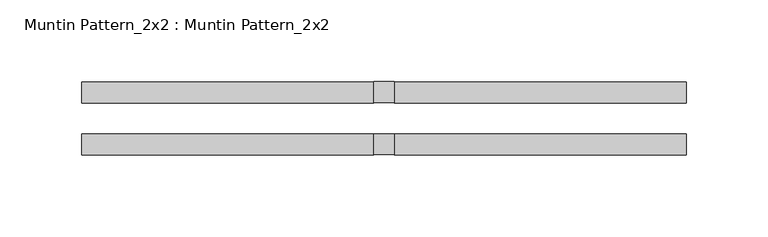
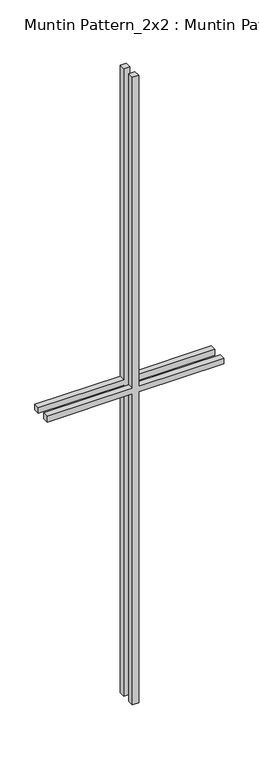
"""IFC4 building model written with IfcOpenShell, lengths in millimetres: proxy geometry, Muntin Pattern_2x2 : Muntin Pattern_2x2."""

from ifc_helpers import new_model, si_unit, frame, origin, place, context, project, spatial, polyline, outline, extrude, source, transform, mapped, element, save


def muntin_pattern_2x2_muntin_pattern_2x2_218eda85(model_context):
    return source(origin(), model_context, "Body", "SweptSolid", [
        extrude(outline(polyline([(698.5, -6.35), (698.5, -184.15), (685.8, -184.15), (685.8, -6.35), (0.0, -6.35), (0.0, 6.35), (685.8, 6.35), (685.8, 184.15), (698.5, 184.15), (698.5, 6.35), (1384.3, 6.35), (1384.3, -6.35), (698.5, -6.35)])), frame((0.0, -22.225, 0.0), z_axis=(0.0, 1.0, 0.0), x_axis=(0.0, 0.0, 1.0)), (0.0, 0.0, 1.0), 12.7),
        extrude(outline(polyline([(698.5, -6.35), (698.5, -184.15), (685.8, -184.15), (685.8, -6.35), (0.0, -6.35), (0.0, 6.35), (685.8, 6.35), (685.8, 184.15), (698.5, 184.15), (698.5, 6.35), (1384.3, 6.35), (1384.3, -6.35), (698.5, -6.35)])), frame((0.0, 9.525, 0.0), z_axis=(0.0, 1.0, 0.0), x_axis=(0.0, 0.0, 1.0)), (0.0, 0.0, 1.0), 12.7),
    ])


if __name__ == "__main__":
    model = new_model("IFC4")
    model_context = context("Model", 3, world=origin())
    ifc_project = project(units=[si_unit("LENGTHUNIT", "METRE", prefix="MILLI")], contexts=[model_context])
    site = spatial("IfcSite", under=ifc_project)
    building = spatial("IfcBuilding", under=site)
    placement = place(None, origin())
    muntin_pattern_2x2_muntin_pattern_2x2_shape = muntin_pattern_2x2_muntin_pattern_2x2_218eda85(model_context)
    element("IfcBuildingElementProxy", 1, Name="Muntin Pattern_2x2 : Muntin Pattern_2x2", ObjectType="Muntin Pattern_2x2 : Muntin Pattern_2x2", at=placement, inside=building, context=model_context, shape_type="MappedRepresentation", body=[
        mapped(muntin_pattern_2x2_muntin_pattern_2x2_shape, transform((0.0, 0.0, 0.0), x_axis=(1.0, 0.0, 0.0), y_axis=(0.0, 1.0, 0.0), z_axis=(0.0, 0.0, 1.0))),
    ])
    save(model, "model.ifc")

# Revit data of these elements
# Type "Muntin Pattern_2x2 : Muntin Pattern_2x2"
#   Width [instance default] = 4' - 0"
#   Thickness = 0' - 0 1/2"
#   Height [instance default] = 4' - 0"
#   Distance = 0' - 0 3/4"
#   Interior Material [instance default] = none
#   Exterior Material [instance default] = none
#   Default Elevation = 0
# Element 1 (IfcBuildingElementProxy, "Muntin Pattern_2x2 : Muntin Pattern_2x2")
#   Width = 1' - 2 1/2"
#   Height = 4' - 6 1/2"
#   Interior Material = Wood - Stained
#   Exterior Material = Clad - White
#   Materials on its faces: "Clad - White", "Wood - Stained"
# Materials
#   "Clad - White": class "Wood", colour RGB 242 242 238, transparency 0, Cost = 0
#   "Wood - Stained": class "Wood", colour RGB 224 178 126, transparency 0, Cost = 0
